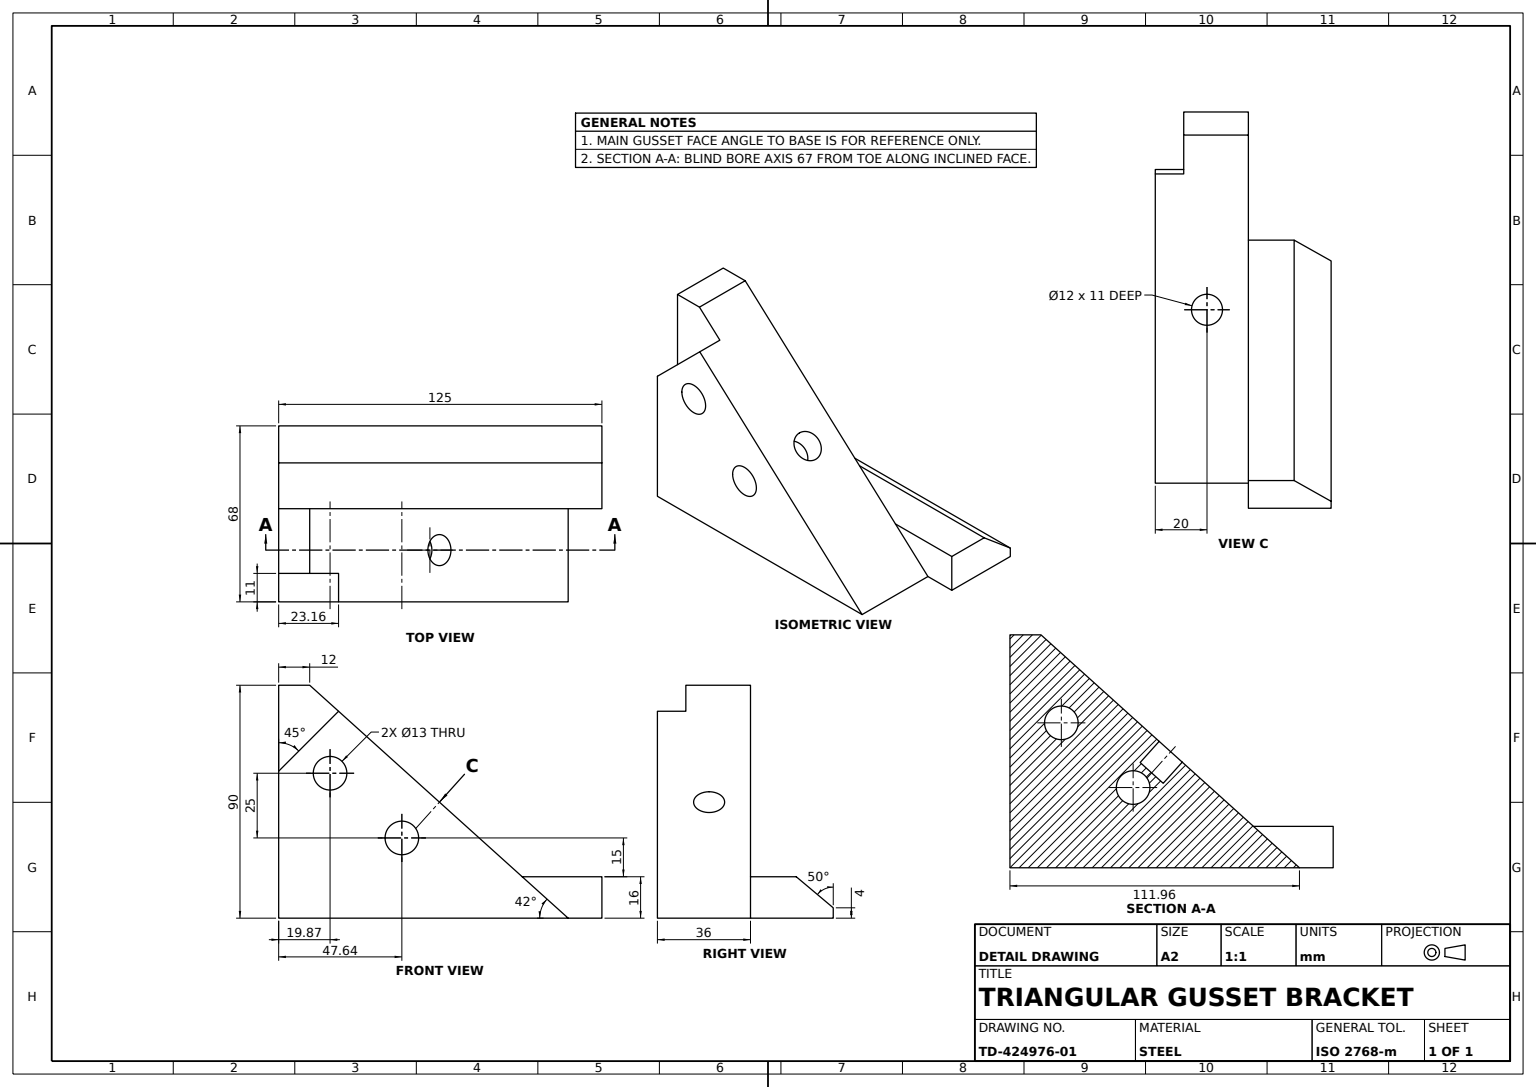
from build123d import *

# Parameters (mm, degrees)
BRACKET_BODY_DEPTH            = 125
PLATE_RELIEF_CUT_DEPTH        = 36
CROSS_HOLES_CUT_11_DEEP_DEPTH = 11
SKETCH3_4_R                   = 6.5
CROSS_HOLES_CUT_36_DEEP_DEPTH = 36
HOLE_12_SKETCH_R              = 6
HOLE_12_DEPTH                 = 11


with BuildPart() as part:
    # Bracket Profile Sketch → Bracket Body (new body)
    with BuildSketch(Plane.XY):
        Polygon((-36, 0), (0, 0), (0, 16), (0, 17.641196013), (0, 90), (-36, 90), align=None)
        Polygon((0, 0), (32, 0), (32, 4), (17.698956889, 16), (0, 16), align=None)
    extrude(amount=BRACKET_BODY_DEPTH)

    # Plate Relief Sketch → Plate Relief Cut (cut)
    with BuildSketch(Plane.ZY.offset(36)):
        Polygon((12, 90), (111.955126335, 0), (125, 0), (125, 90), align=None)
    extrude(amount=-PLATE_RELIEF_CUT_DEPTH, mode=Mode.SUBTRACT)

    # Cross Holes Sketch → Cross Holes Cut 11 Deep (cut)
    with BuildSketch(Plane.ZY.offset(36)):
        Polygon((-5.668578971, 51.118217594), (-13.477683521, 103.633494759), (27.976080454, 91.378914898), (26.142244571, 82.929041136), align=None)
    extrude(amount=-CROSS_HOLES_CUT_11_DEEP_DEPTH, mode=Mode.SUBTRACT)

    # Sketch3_4 → Cross Holes Cut 36 Deep (cut)
    with BuildSketch(Plane.ZY.offset(36)):
        with Locations((19.871294507, 56)):
            Circle(SKETCH3_4_R)
        with Locations((47.636607378, 31)):
            Circle(SKETCH3_4_R)
    extrude(amount=-CROSS_HOLES_CUT_36_DEEP_DEPTH, mode=Mode.SUBTRACT)

    # Hole _12 Sketch → Hole _12 (cut)
    with BuildSketch(Plane(origin=(0, 55.670912219, 50.126314512), x_dir=(1, 0, 0), z_dir=(0, 0.7431448254773981, 0.669130606358854))):
        with Locations(Location((-16, -16.198872821, 0), (0, 0, 270))):
            Circle(HOLE_12_SKETCH_R)
    extrude(amount=-HOLE_12_DEPTH, mode=Mode.SUBTRACT)


solid = part.part
